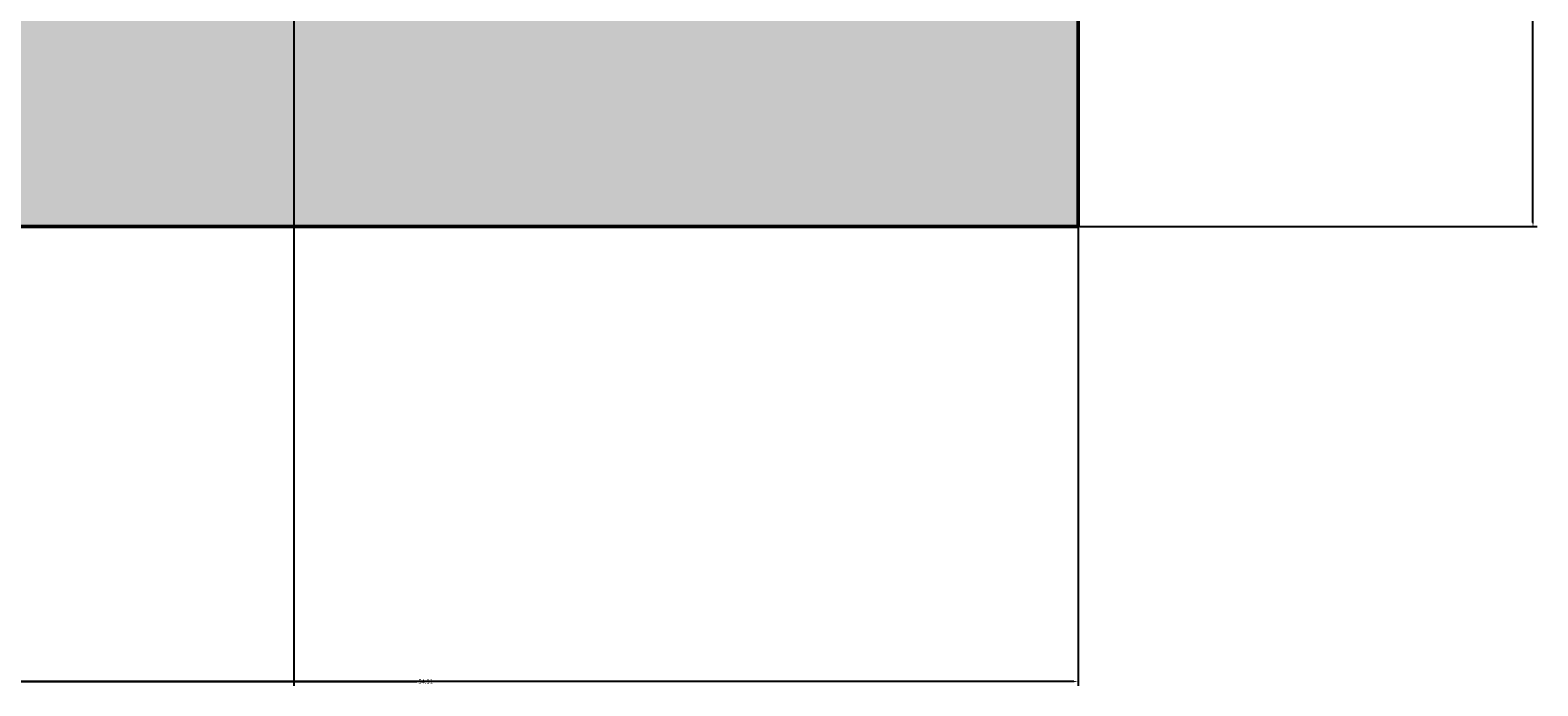
# Model space of a CAD drawing. Units: inches. Extents: x 2307 to 2544, y 2171 to 2540.
# Tile 10 of 52: x 2481 to 2544, y 2171 to 2199. Entities that reach past the tile are written whole.
import ezdxf

# ---------------------------------------------------------------- set-up
doc = ezdxf.new("R2010")
doc.units = ezdxf.units.IN
doc.layers.add('A-ANNO-DIMS', color=2, linetype='Continuous', lineweight=18)
doc.layers.add('A-WALL', color=7, linetype='Continuous', lineweight=50)
doc.layers.add('A-WALL-PATT', color=18, linetype='Continuous', lineweight=13, true_color=0x000000)
doc.styles.get("Standard").update_dxf_attribs({"font": 'arial.ttf'})
doc.dimstyles.get("Standard").update_dxf_attribs({"dimtxt": 0.18, "dimasz": 0.18, "dimexe": 0.18, "dimexo": 0.0625, "dimgap": 0.09, "dimtad": 0, "dimtih": 1, "dimtoh": 1, "dimdec": 4, "dimzin": 0, "dimdsep": 46, "dimtxsty": 'Standard', "dimcen": 0.09, "dimadec": 0, "dimazin": 0, "dimtfac": 1, "dimtdec": 4, "dimtofl": 0, "dimtmove": 0, "dimatfit": 3, "dimfxl": 1, "dimtolj": 1, "dimtzin": 0, "dimarcsym": 0})

# ---------------------------------------------------------------- blocks, each defined once
blk = doc.blocks.new('*D36')
at = {"layer": 'A-ANNO-DIMS', "color": 0, "lineweight": -2, "transparency": 16777216}
for p, q in [((2326.696, 2190.447), (2326.696, 2171.18)), ((2524.696, 2190.447), (2524.696, 2171.18)), ((2326.876, 2171.36), (2425.415, 2171.36)), ((2524.516, 2171.36), (2425.976, 2171.36))]:
    blk.add_line(p, q, dxfattribs=at)
at = {"layer": 'A-ANNO-DIMS', "color": 0, "transparency": 16777216}
for points in [[(2326.876, 2171.39), (2326.876, 2171.33), (2326.696, 2171.36)], [(2524.516, 2171.39), (2524.516, 2171.33), (2524.696, 2171.36)]]:
    blk.add_solid(points, dxfattribs=at)
at = {"layer": 'Defpoints', "color": 0, "transparency": 16777216}
for p in [(2326.696, 2190.51), (2524.696, 2190.51), (2524.696, 2171.36)]:
    blk.add_point(p, dxfattribs=at)
at = {"layer": 'A-ANNO-DIMS', "color": 0, "transparency": 16777216, "insert": (2425.696, 2171.36), "char_height": 0.18, "attachment_point": 5}
blk.add_mtext('\\A1;198', dxfattribs=at)
blk = doc.blocks.new('*D37')
at = {"layer": 'A-ANNO-DIMS', "color": 0, "lineweight": -2, "transparency": 16777216}
for p, q in [((2524.758, 2520.51), (2544.026, 2520.51)), ((2543.846, 2520.33), (2543.846, 2355.692)), ((2543.846, 2190.69), (2543.846, 2355.328)), ((2524.758, 2190.51), (2544.026, 2190.51))]:
    blk.add_line(p, q, dxfattribs=at)
at = {"layer": 'A-ANNO-DIMS', "color": 0, "transparency": 16777216}
for points in [[(2543.816, 2520.33), (2543.876, 2520.33), (2543.846, 2520.51)], [(2543.816, 2190.69), (2543.876, 2190.69), (2543.846, 2190.51)]]:
    blk.add_solid(points, dxfattribs=at)
at = {"layer": 'Defpoints', "color": 0, "transparency": 16777216}
for p in [(2524.696, 2520.51), (2543.846, 2520.51), (2524.696, 2190.51)]:
    blk.add_point(p, dxfattribs=at)
at = {"layer": 'A-ANNO-DIMS', "color": 0, "transparency": 16777216, "insert": (2543.846, 2355.51), "char_height": 0.18, "attachment_point": 5}
blk.add_mtext('\\A1;330', dxfattribs=at)
blk = doc.blocks.new('*D39')
at = {"layer": 'A-ANNO-DIMS', "color": 0, "lineweight": -2, "transparency": 16777216}
for p, q in [((2469.783, 2190.447), (2469.783, 2171.18)), ((2524.696, 2190.447), (2524.696, 2171.18)), ((2469.963, 2171.36), (2496.863, 2171.36)), ((2524.516, 2171.36), (2497.616, 2171.36))]:
    blk.add_line(p, q, dxfattribs=at)
at = {"layer": 'A-ANNO-DIMS', "color": 0, "transparency": 16777216}
for points in [[(2469.963, 2171.39), (2469.963, 2171.33), (2469.783, 2171.36)], [(2524.516, 2171.39), (2524.516, 2171.33), (2524.696, 2171.36)]]:
    blk.add_solid(points, dxfattribs=at)
at = {"layer": 'Defpoints', "color": 0, "transparency": 16777216}
for p in [(2469.783, 2190.51), (2524.696, 2190.51), (2524.696, 2171.36)]:
    blk.add_point(p, dxfattribs=at)
at = {"layer": 'A-ANNO-DIMS', "color": 0, "transparency": 16777216, "insert": (2497.24, 2171.36), "char_height": 0.18, "attachment_point": 5}
blk.add_mtext('\\A1;54.91', dxfattribs=at)
blk = doc.blocks.new('*D54')
at = {"layer": 'A-ANNO-DIMS', "color": 0, "lineweight": -2, "transparency": 16777216}
for p, q in [((2461.696, 2435.447), (2461.696, 2171.18)), ((2491.696, 2435.447), (2491.696, 2171.18)), ((2461.876, 2171.36), (2476.477, 2171.36)), ((2491.516, 2171.36), (2476.914, 2171.36))]:
    blk.add_line(p, q, dxfattribs=at)
at = {"layer": 'A-ANNO-DIMS', "color": 0, "transparency": 16777216}
for points in [[(2461.876, 2171.39), (2461.876, 2171.33), (2461.696, 2171.36)], [(2491.516, 2171.39), (2491.516, 2171.33), (2491.696, 2171.36)]]:
    blk.add_solid(points, dxfattribs=at)
at = {"layer": 'Defpoints', "color": 0, "transparency": 16777216}
for p in [(2461.696, 2435.51), (2491.696, 2435.51), (2491.696, 2171.36)]:
    blk.add_point(p, dxfattribs=at)
at = {"layer": 'A-ANNO-DIMS', "color": 0, "transparency": 16777216, "insert": (2476.696, 2171.36), "char_height": 0.18, "attachment_point": 5}
blk.add_mtext('\\A1;30', dxfattribs=at)

msp = doc.modelspace()

# ---------------------------------------------------------------- hatches: boundary and pattern name
at = {"layer": 'A-WALL-PATT'}
h = msp.add_hatch(color=256, dxfattribs=at)
h.dxf.hatch_style = 1
h.paths.add_polyline_path([(2433.6935, 2199.5096), (2415.6423, 2199.5096), (2415.6423, 2190.5096), (2433.7832, 2190.5096)], flags=17)
h.paths.add_polyline_path([(2367.6423, 2199.5096), (2335.6958, 2199.5096), (2335.6958, 2307.3983), (2326.6958, 2307.3983), (2326.6958, 2190.5096), (2367.6423, 2190.5096)])
h.paths.add_polyline_path([(2524.6958, 2520.5096), (2496.7832, 2520.5096), (2496.7832, 2515.5149), (2472.7832, 2515.5149), (2472.7832, 2520.5096), (2415.4028, 2520.5096), (2415.4028, 2511.5096), (2451.6958, 2511.5096), (2451.6958, 2439.5096), (2451.6958, 2391.5096), (2445.6958, 2391.5096), (2445.6958, 2387.5096), (2455.6958, 2387.5096), (2455.6958, 2435.5096), (2461.6958, 2435.5096), (2461.6958, 2439.5096), (2455.6958, 2439.5096), (2455.6958, 2511.5096), (2515.6958, 2511.5096), (2515.6958, 2439.5096), (2491.6958, 2439.5096), (2491.6958, 2435.5096), (2515.6958, 2435.5096), (2515.6958, 2319.5096), (2451.6958, 2319.5096), (2451.6958, 2281.5096), (2481.6958, 2281.5096), (2481.6958, 2225.5096), (2485.6958, 2225.5096), (2485.6958, 2285.5096), (2455.6958, 2285.5096), (2455.6958, 2315.5096), (2515.6958, 2315.5096), (2515.6958, 2199.5096), (2469.6952, 2199.5096), (2469.785, 2190.5096), (2524.6958, 2190.5096)])

# ---------------------------------------------------------------- linework, layer by layer
at = {"layer": 'A-WALL'}
msp.add_lwpolyline([(2433.7832, 2190.5096), (2326.6958, 2190.5096), (2326.6958, 2520.5096), (2524.6958, 2520.5096), (2524.6958, 2190.5096), (2469.785, 2190.5096)], dxfattribs=at)

# ---------------------------------------------------------------- dimensions: what is measured, and where the dimension line sits
at = {"layer": 'A-ANNO-DIMS'}
dim = msp.add_linear_dim(base=(2543.8458, 2520.5096), p1=(2524.6958, 2190.5096), p2=(2524.6958, 2520.5096), angle=90, dimstyle='Standard', override={"dimdec": 0, "dimlfac": 1, "dimrnd": 0, "dimzin": 0, "dimdsep": 46, "dimlunit": 2}, dxfattribs=at)
dim.commit()
dim.dimension.update_dxf_attribs({"geometry": '*D37', "text_midpoint": (2543.8458, 2355.5096)})
for base, p1, p2, override, picture, middle in [((2491.6958, 2171.3596), (2461.6958, 2435.5096), (2491.6958, 2435.5096), {"dimdec": 0, "dimlfac": 1, "dimrnd": 0, "dimzin": 0, "dimdsep": 46, "dimlunit": 2}, '*D54', (2476.6958, 2171.3596)), ((2524.6958, 2171.3596), (2326.6958, 2190.5096), (2524.6958, 2190.5096), {"dimdec": 0, "dimlfac": 1, "dimrnd": 0, "dimzin": 0, "dimdsep": 46, "dimlunit": 2}, '*D36', (2425.6958, 2171.3596)), ((2524.6958, 2171.3596), (2469.7832, 2190.5096), (2524.6958, 2190.5096), {"dimdec": 2, "dimlfac": 1, "dimrnd": 0, "dimzin": 0, "dimdsep": 46, "dimlunit": 2}, '*D39', (2497.2395, 2171.3596))]:
    dim = msp.add_linear_dim(base=base, p1=p1, p2=p2, dimstyle='Standard', override=override, dxfattribs=at)
    dim.commit()
    dim.dimension.update_dxf_attribs({"geometry": picture, "text_midpoint": middle})

doc.saveas('drawing.dxf')
